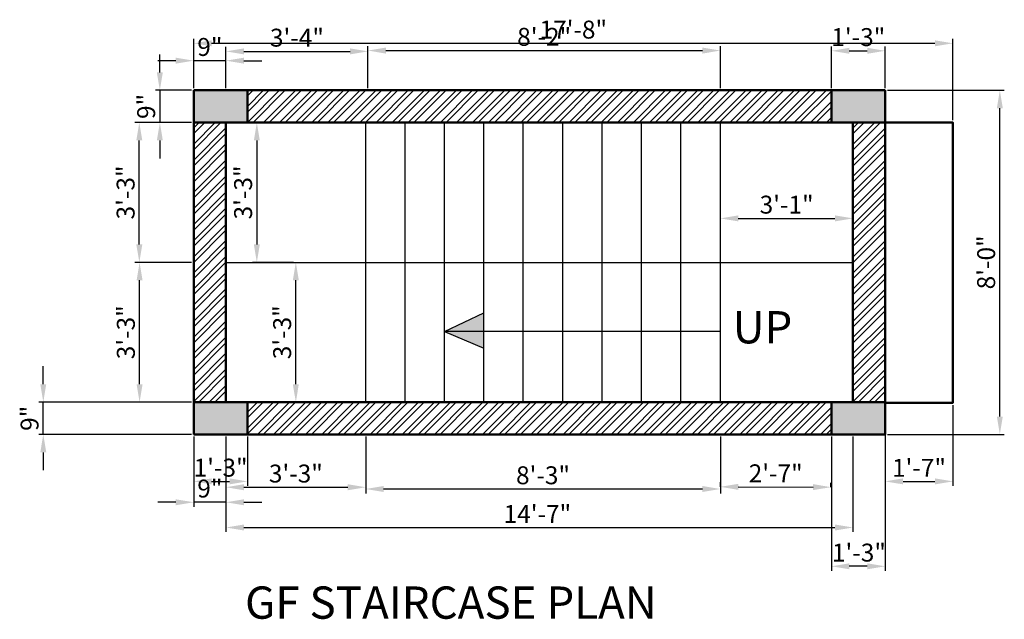
# Model space of a CAD drawing. Units: inches. Extents: x 1925 to 2200, y 918 to 1361.
# Tile 1 of 2: x 1925 to 2200, y 918 to 1085. Entities that reach past the tile are written whole.
import ezdxf

# ---------------------------------------------------------------- set-up
doc = ezdxf.new("R2010")
doc.units = ezdxf.units.IN
for name, color, linetype, lineweight in [('A-ANNO-DIMS', 2, 'Continuous', 18), ('A-ANNO-TEXT', 7, 'Continuous', 25), ('A-FLOR-STRS', 4, 'Continuous', 25), ('A-WALL', 7, 'Continuous', 50), ('A-WALL-PATT', 8, 'Continuous', 13), ('S-COLS-PATT', 1, 'Continuous', 13)]:
    doc.layers.add(name, color=color, linetype=linetype, lineweight=lineweight)
doc.styles.get("Standard").update_dxf_attribs({"font": 'arial.ttf'})
doc.dimstyles.new('ISO-25', dxfattribs={"dimtxt": 5, "dimasz": 5, "dimexe": 1.25, "dimexo": 0.625, "dimtad": 1, "dimdec": 0, "dimlunit": 3, "dimtxsty": 'Standard', "dimcen": 2.5, "dimadec": 0, "dimazin": 0, "dimtfac": 1, "dimtdec": 0, "dimtmove": 0, "dimatfit": 3, "dimfxl": 1, "dimarcsym": 0})
pattern_1 = [(45, (0, 0), (-2.245064, 2.245064), []), (45, (0, 1.5875), (-2.245064, 2.245064), [])]

# ---------------------------------------------------------------- blocks, each defined once
blk = doc.blocks.new('*D1')
at = {"layer": 'A-ANNO-DIMS', "color": 0, "lineweight": -2, "transparency": 16777216}
for p, q in [((2120.9, 1018.14), (2120.9, 1031.03)), ((2157.9, 1018.14), (2157.9, 1031.03)), ((2125.9, 1029.78), (2152.9, 1029.78))]:
    blk.add_line(p, q, dxfattribs=at)
at = {"layer": 'A-ANNO-DIMS', "color": 0, "transparency": 16777216}
for points in [[(2125.9, 1030.61), (2125.9, 1028.94), (2120.9, 1029.78)], [(2152.9, 1030.61), (2152.9, 1028.94), (2157.9, 1029.78)]]:
    blk.add_solid(points, dxfattribs=at)
at = {"layer": 'Defpoints', "color": 0, "transparency": 16777216}
for p in [(2157.9, 1029.78), (2120.9, 1017.51), (2157.9, 1017.51)]:
    blk.add_point(p, dxfattribs=at)
at = {"layer": 'A-ANNO-DIMS', "color": 0, "transparency": 16777216, "insert": (2139.4, 1032.96), "char_height": 5, "attachment_point": 5}
blk.add_mtext('3\'-1"', dxfattribs=at)
blk = doc.blocks.new('*D2')
at = {"layer": 'A-ANNO-DIMS', "color": 0, "lineweight": -2, "transparency": 16777216}
for p, q in [((1973.9, 1066.14), (1973.9, 1075.02)), ((1982.9, 1066.14), (1982.9, 1075.02)), ((1968.9, 1073.77), (1963.9, 1073.77)), ((1982.9, 1073.77), (1973.9, 1073.77)), ((1987.9, 1073.77), (1992.9, 1073.77))]:
    blk.add_line(p, q, dxfattribs=at)
at = {"layer": 'A-ANNO-DIMS', "color": 0, "transparency": 16777216}
for points in [[(1968.9, 1074.6), (1968.9, 1072.94), (1973.9, 1073.77)], [(1987.9, 1074.6), (1987.9, 1072.94), (1982.9, 1073.77)]]:
    blk.add_solid(points, dxfattribs=at)
at = {"layer": 'Defpoints', "color": 0, "transparency": 16777216}
for p in [(1973.9, 1073.77), (1973.9, 1065.51), (1982.9, 1065.51)]:
    blk.add_point(p, dxfattribs=at)
at = {"layer": 'A-ANNO-DIMS', "color": 0, "transparency": 16777216, "insert": (1978.4, 1076.95), "char_height": 5, "attachment_point": 5}
blk.add_mtext('9"', dxfattribs=at)
blk = doc.blocks.new('*D3')
at = {"layer": 'A-ANNO-DIMS', "color": 0, "lineweight": -2, "transparency": 16777216}
for p, q in [((1931.9, 983.51), (1931.9, 988.51)), ((1973.27, 978.51), (1930.65, 978.51)), ((1931.9, 969.51), (1931.9, 978.51)), ((1973.27, 969.51), (1930.65, 969.51)), ((1931.9, 964.51), (1931.9, 959.51))]:
    blk.add_line(p, q, dxfattribs=at)
at = {"layer": 'A-ANNO-DIMS', "color": 0, "transparency": 16777216}
for points in [[(1931.07, 983.51), (1932.73, 983.51), (1931.9, 978.51)], [(1931.07, 964.51), (1932.73, 964.51), (1931.9, 969.51)]]:
    blk.add_solid(points, dxfattribs=at)
at = {"layer": 'Defpoints', "color": 0, "transparency": 16777216}
for p in [(1931.9, 978.51), (1973.9, 978.51), (1973.9, 969.51)]:
    blk.add_point(p, dxfattribs=at)
at = {"layer": 'A-ANNO-DIMS', "color": 0, "transparency": 16777216, "insert": (1928.72, 974.01), "char_height": 5, "attachment_point": 5, "rotation": 90}
blk.add_mtext('9"', dxfattribs=at)
blk = doc.blocks.new('*D4')
at = {"layer": 'A-ANNO-DIMS', "color": 0, "lineweight": -2, "transparency": 16777216}
for p, q in [((1964.44, 1070.51), (1964.44, 1075.51)), ((1973.27, 1065.51), (1963.19, 1065.51)), ((1964.44, 1065.51), (1964.44, 1056.51)), ((1973.27, 1056.51), (1963.19, 1056.51)), ((1964.44, 1051.51), (1964.44, 1046.51))]:
    blk.add_line(p, q, dxfattribs=at)
at = {"layer": 'A-ANNO-DIMS', "color": 0, "transparency": 16777216}
for points in [[(1963.6, 1070.51), (1965.27, 1070.51), (1964.44, 1065.51)], [(1963.6, 1051.51), (1965.27, 1051.51), (1964.44, 1056.51)]]:
    blk.add_solid(points, dxfattribs=at)
at = {"layer": 'Defpoints', "color": 0, "transparency": 16777216}
for p in [(1973.9, 1065.51), (1964.44, 1056.51), (1973.9, 1056.51)]:
    blk.add_point(p, dxfattribs=at)
at = {"layer": 'A-ANNO-DIMS', "color": 0, "transparency": 16777216, "insert": (1961.26, 1061.01), "char_height": 5, "attachment_point": 5, "rotation": 90}
blk.add_mtext('9"', dxfattribs=at)
blk = doc.blocks.new('*D5')
at = {"layer": 'A-ANNO-DIMS', "color": 0, "lineweight": -2, "transparency": 16777216}
for p, q in [((1973.9, 968.89), (1973.9, 949.34)), ((1982.9, 968.89), (1982.9, 949.34)), ((1968.9, 950.59), (1963.9, 950.59)), ((1982.9, 950.59), (1973.9, 950.59)), ((1987.9, 950.59), (1992.9, 950.59))]:
    blk.add_line(p, q, dxfattribs=at)
at = {"layer": 'A-ANNO-DIMS', "color": 0, "transparency": 16777216}
for points in [[(1968.9, 951.42), (1968.9, 949.75), (1973.9, 950.59)], [(1987.9, 951.42), (1987.9, 949.75), (1982.9, 950.59)]]:
    blk.add_solid(points, dxfattribs=at)
at = {"layer": 'Defpoints', "color": 0, "transparency": 16777216}
for p in [(1973.9, 969.51), (1982.9, 969.51), (1973.9, 950.59)]:
    blk.add_point(p, dxfattribs=at)
at = {"layer": 'A-ANNO-DIMS', "color": 0, "transparency": 16777216, "insert": (1978.4, 953.77), "char_height": 5, "attachment_point": 5}
blk.add_mtext('9"', dxfattribs=at)
blk = doc.blocks.new('*D6')
at = {"layer": 'A-ANNO-DIMS', "color": 0, "lineweight": -2, "transparency": 16777216}
for p, q in [((1982.9, 968.89), (1982.9, 942.3)), ((2157.9, 968.89), (2157.9, 942.3)), ((1987.9, 943.55), (2152.9, 943.55))]:
    blk.add_line(p, q, dxfattribs=at)
at = {"layer": 'A-ANNO-DIMS', "color": 0, "transparency": 16777216}
for points in [[(1987.9, 944.38), (1987.9, 942.72), (1982.9, 943.55)], [(2152.9, 944.38), (2152.9, 942.72), (2157.9, 943.55)]]:
    blk.add_solid(points, dxfattribs=at)
at = {"layer": 'Defpoints', "color": 0, "transparency": 16777216}
for p in [(1982.9, 969.51), (2157.9, 969.51), (2157.9, 943.55)]:
    blk.add_point(p, dxfattribs=at)
at = {"layer": 'A-ANNO-DIMS', "color": 0, "transparency": 16777216, "insert": (2069.82, 946.68), "char_height": 5, "attachment_point": 5}
blk.add_mtext('14\'-7"', dxfattribs=at)
blk = doc.blocks.new('*D7')
at = {"layer": 'A-ANNO-DIMS', "color": 0, "lineweight": -2, "transparency": 16777216}
for p, q in [((1973.27, 1017.51), (1957.53, 1017.51)), ((1958.78, 983.51), (1958.78, 1012.51)), ((1973.27, 978.51), (1957.53, 978.51))]:
    blk.add_line(p, q, dxfattribs=at)
at = {"layer": 'A-ANNO-DIMS', "color": 0, "transparency": 16777216}
for points in [[(1957.95, 1012.51), (1959.61, 1012.51), (1958.78, 1017.51)], [(1957.95, 983.51), (1959.61, 983.51), (1958.78, 978.51)]]:
    blk.add_solid(points, dxfattribs=at)
at = {"layer": 'Defpoints', "color": 0, "transparency": 16777216}
for p in [(1958.78, 1017.51), (1973.9, 1017.51), (1973.9, 978.51)]:
    blk.add_point(p, dxfattribs=at)
at = {"layer": 'A-ANNO-DIMS', "color": 0, "transparency": 16777216, "insert": (1955.6, 998.01), "char_height": 5, "attachment_point": 5, "rotation": 90}
blk.add_mtext('3\'-3"', dxfattribs=at)
blk = doc.blocks.new('*D8')
at = {"layer": 'A-ANNO-DIMS', "color": 0, "lineweight": -2, "transparency": 16777216}
for p, q in [((1973.27, 1056.51), (1957.46, 1056.51)), ((1958.71, 1022.51), (1958.71, 1051.51)), ((1973.27, 1017.51), (1957.46, 1017.51))]:
    blk.add_line(p, q, dxfattribs=at)
at = {"layer": 'A-ANNO-DIMS', "color": 0, "transparency": 16777216}
for points in [[(1957.87, 1051.51), (1959.54, 1051.51), (1958.71, 1056.51)], [(1957.87, 1022.51), (1959.54, 1022.51), (1958.71, 1017.51)]]:
    blk.add_solid(points, dxfattribs=at)
at = {"layer": 'Defpoints', "color": 0, "transparency": 16777216}
for p in [(1958.71, 1056.51), (1973.9, 1056.51), (1973.9, 1017.51)]:
    blk.add_point(p, dxfattribs=at)
at = {"layer": 'A-ANNO-DIMS', "color": 0, "transparency": 16777216, "insert": (1955.53, 1037.01), "char_height": 5, "attachment_point": 5, "rotation": 90}
blk.add_mtext('3\'-3"', dxfattribs=at)
blk = doc.blocks.new('*D9')
at = {"layer": 'A-ANNO-DIMS', "color": 0, "lineweight": -2, "transparency": 16777216}
for p, q in [((1982.9, 1066.14), (1982.9, 1077.61)), ((2022.53, 1066.14), (2022.53, 1077.61)), ((1987.9, 1076.36), (2017.53, 1076.36))]:
    blk.add_line(p, q, dxfattribs=at)
at = {"layer": 'A-ANNO-DIMS', "color": 0, "transparency": 16777216}
for points in [[(1987.9, 1077.2), (1987.9, 1075.53), (1982.9, 1076.36)], [(2017.53, 1077.2), (2017.53, 1075.53), (2022.53, 1076.36)]]:
    blk.add_solid(points, dxfattribs=at)
at = {"layer": 'Defpoints', "color": 0, "transparency": 16777216}
for p in [(2022.53, 1076.36), (1982.9, 1065.51), (2022.53, 1065.51)]:
    blk.add_point(p, dxfattribs=at)
at = {"layer": 'A-ANNO-DIMS', "color": 0, "transparency": 16777216, "insert": (2002.71, 1079.54), "char_height": 5, "attachment_point": 5}
blk.add_mtext('3\'-4"', dxfattribs=at)
blk = doc.blocks.new('*D10')
at = {"layer": 'A-ANNO-DIMS', "color": 0, "lineweight": -2, "transparency": 16777216}
for p, q in [((2022.53, 1066.14), (2022.53, 1077.84)), ((2120.9, 1066.14), (2120.9, 1077.84)), ((2027.53, 1076.59), (2115.9, 1076.59))]:
    blk.add_line(p, q, dxfattribs=at)
at = {"layer": 'A-ANNO-DIMS', "color": 0, "transparency": 16777216}
for points in [[(2027.53, 1077.42), (2027.53, 1075.75), (2022.53, 1076.59)], [(2115.9, 1077.42), (2115.9, 1075.75), (2120.9, 1076.59)]]:
    blk.add_solid(points, dxfattribs=at)
at = {"layer": 'Defpoints', "color": 0, "transparency": 16777216}
for p in [(2120.9, 1076.59), (2022.53, 1065.51), (2120.9, 1065.51)]:
    blk.add_point(p, dxfattribs=at)
at = {"layer": 'A-ANNO-DIMS', "color": 0, "transparency": 16777216, "insert": (2071.71, 1079.77), "char_height": 5, "attachment_point": 5}
blk.add_mtext('8\'-2"', dxfattribs=at)
blk = doc.blocks.new('*D11')
at = {"layer": 'A-ANNO-DIMS', "color": 0, "lineweight": -2, "transparency": 16777216}
for p, q in [((2003.02, 1017.51), (2003.65, 1017.51)), ((2002.4, 983.51), (2002.4, 1012.51)), ((2003.02, 978.51), (2003.65, 978.51))]:
    blk.add_line(p, q, dxfattribs=at)
at = {"layer": 'A-ANNO-DIMS', "color": 0, "transparency": 16777216}
for points in [[(2001.56, 1012.51), (2003.23, 1012.51), (2002.4, 1017.51)], [(2001.56, 983.51), (2003.23, 983.51), (2002.4, 978.51)]]:
    blk.add_solid(points, dxfattribs=at)
at = {"layer": 'Defpoints', "color": 0, "transparency": 16777216}
for p in [(2002.4, 1017.51), (2002.4, 1017.51), (2002.4, 978.51)]:
    blk.add_point(p, dxfattribs=at)
at = {"layer": 'A-ANNO-DIMS', "color": 0, "transparency": 16777216, "insert": (1999.22, 998.01), "char_height": 5, "attachment_point": 5, "rotation": 90}
blk.add_mtext('3\'-3"', dxfattribs=at)
blk = doc.blocks.new('*D12')
at = {"layer": 'A-ANNO-DIMS', "color": 0, "lineweight": -2, "transparency": 16777216}
for p, q in [((2001.77, 1056.51), (1990.26, 1056.51)), ((1991.51, 1051.51), (1991.51, 1022.51)), ((2001.77, 1017.51), (1990.26, 1017.51))]:
    blk.add_line(p, q, dxfattribs=at)
at = {"layer": 'A-ANNO-DIMS', "color": 0, "transparency": 16777216}
for points in [[(1990.68, 1051.51), (1992.34, 1051.51), (1991.51, 1056.51)], [(1990.68, 1022.51), (1992.34, 1022.51), (1991.51, 1017.51)]]:
    blk.add_solid(points, dxfattribs=at)
at = {"layer": 'Defpoints', "color": 0, "transparency": 16777216}
for p in [(2002.4, 1056.51), (1991.51, 1017.51), (2002.4, 1017.51)]:
    blk.add_point(p, dxfattribs=at)
at = {"layer": 'A-ANNO-DIMS', "color": 0, "transparency": 16777216, "insert": (1988.33, 1037.01), "char_height": 5, "attachment_point": 5, "rotation": 90}
blk.add_mtext('3\'-3"', dxfattribs=at)
blk = doc.blocks.new('*D13')
at = {"layer": 'A-ANNO-DIMS', "color": 0, "lineweight": -2, "transparency": 16777216}
for p, q in [((2151.9, 1066.14), (2151.9, 1077.77)), ((2166.9, 1066.14), (2166.9, 1077.77)), ((2156.9, 1076.52), (2161.9, 1076.52))]:
    blk.add_line(p, q, dxfattribs=at)
at = {"layer": 'A-ANNO-DIMS', "color": 0, "transparency": 16777216}
for points in [[(2156.9, 1077.36), (2156.9, 1075.69), (2151.9, 1076.52)], [(2161.9, 1077.36), (2161.9, 1075.69), (2166.9, 1076.52)]]:
    blk.add_solid(points, dxfattribs=at)
at = {"layer": 'Defpoints', "color": 0, "transparency": 16777216}
for p in [(2166.9, 1076.52), (2151.9, 1065.51), (2166.9, 1065.51)]:
    blk.add_point(p, dxfattribs=at)
at = {"layer": 'A-ANNO-DIMS', "color": 0, "transparency": 16777216, "insert": (2159.4, 1079.7), "char_height": 5, "attachment_point": 5}
blk.add_mtext('1\'-3"', dxfattribs=at)
blk = doc.blocks.new('*D14')
at = {"layer": 'A-ANNO-DIMS', "color": 0, "lineweight": -2, "transparency": 16777216}
for p, q in [((2151.9, 968.89), (2151.9, 931.47)), ((2166.9, 968.89), (2166.9, 931.47)), ((2161.9, 932.72), (2156.9, 932.72))]:
    blk.add_line(p, q, dxfattribs=at)
at = {"layer": 'A-ANNO-DIMS', "color": 0, "transparency": 16777216}
for points in [[(2156.9, 933.56), (2156.9, 931.89), (2151.9, 932.72)], [(2161.9, 933.56), (2161.9, 931.89), (2166.9, 932.72)]]:
    blk.add_solid(points, dxfattribs=at)
at = {"layer": 'Defpoints', "color": 0, "transparency": 16777216}
for p in [(2151.9, 969.51), (2166.9, 969.51), (2151.9, 932.72)]:
    blk.add_point(p, dxfattribs=at)
at = {"layer": 'A-ANNO-DIMS', "color": 0, "transparency": 16777216, "insert": (2159.58, 935.9), "char_height": 5, "attachment_point": 5}
blk.add_mtext('1\'-3"', dxfattribs=at)
blk = doc.blocks.new('*D15')
at = {"layer": 'A-ANNO-DIMS', "color": 0, "lineweight": -2, "transparency": 16777216}
for p, q in [((1982.9, 968.89), (1982.9, 953.53)), ((2021.9, 968.89), (2021.9, 953.53)), ((1987.9, 954.78), (2016.9, 954.78))]:
    blk.add_line(p, q, dxfattribs=at)
at = {"layer": 'A-ANNO-DIMS', "color": 0, "transparency": 16777216}
for points in [[(1987.9, 955.61), (1987.9, 953.94), (1982.9, 954.78)], [(2016.9, 955.61), (2016.9, 953.94), (2021.9, 954.78)]]:
    blk.add_solid(points, dxfattribs=at)
at = {"layer": 'Defpoints', "color": 0, "transparency": 16777216}
for p in [(1982.9, 969.51), (2021.9, 969.51), (2021.9, 954.78)]:
    blk.add_point(p, dxfattribs=at)
at = {"layer": 'A-ANNO-DIMS', "color": 0, "transparency": 16777216, "insert": (2002.4, 957.95), "char_height": 5, "attachment_point": 5}
blk.add_mtext('3\'-3"', dxfattribs=at)
blk = doc.blocks.new('*D16')
at = {"layer": 'A-ANNO-DIMS', "color": 0, "lineweight": -2, "transparency": 16777216}
for p, q in [((2021.9, 968.89), (2021.9, 953.04)), ((2120.9, 968.89), (2120.9, 953.04)), ((2026.9, 954.29), (2115.9, 954.29))]:
    blk.add_line(p, q, dxfattribs=at)
at = {"layer": 'A-ANNO-DIMS', "color": 0, "transparency": 16777216}
for points in [[(2026.9, 955.12), (2026.9, 953.45), (2021.9, 954.29)], [(2115.9, 955.12), (2115.9, 953.45), (2120.9, 954.29)]]:
    blk.add_solid(points, dxfattribs=at)
at = {"layer": 'Defpoints', "color": 0, "transparency": 16777216}
for p in [(2021.9, 969.51), (2120.9, 969.51), (2120.9, 954.29)]:
    blk.add_point(p, dxfattribs=at)
at = {"layer": 'A-ANNO-DIMS', "color": 0, "transparency": 16777216, "insert": (2071.4, 957.47), "char_height": 5, "attachment_point": 5}
blk.add_mtext('8\'-3"', dxfattribs=at)
blk = doc.blocks.new('*D17')
at = {"layer": 'A-ANNO-DIMS', "color": 0, "lineweight": -2, "transparency": 16777216}
for p, q in [((2120.9, 954.91), (2120.9, 956.15)), ((2125.9, 954.88), (2146.77, 954.82)), ((2151.77, 954.81), (2151.77, 956.05))]:
    blk.add_line(p, q, dxfattribs=at)
at = {"layer": 'A-ANNO-DIMS', "color": 0, "transparency": 16777216}
for points in [[(2125.9, 955.72), (2125.89, 954.05), (2120.9, 954.9)], [(2146.77, 955.65), (2146.77, 953.98), (2151.77, 954.8)]]:
    blk.add_solid(points, dxfattribs=at)
at = {"layer": 'Defpoints', "color": 0, "transparency": 16777216}
for p in [(2120.9, 954.29), (2151.77, 954.8), (2151.77, 954.19)]:
    blk.add_point(p, dxfattribs=at)
at = {"layer": 'A-ANNO-DIMS', "color": 0, "transparency": 16777216, "insert": (2136.34, 957.99), "char_height": 5, "attachment_point": 5, "rotation": 359.8217}
blk.add_mtext('2\'-7"', dxfattribs=at)
blk = doc.blocks.new('*D38')
at = {"layer": 'A-ANNO-DIMS', "color": 0, "lineweight": -2, "transparency": 16777216}
for p, q in [((1973.9, 1066.14), (1973.9, 1079.86)), ((1978.9, 1078.61), (2180.81, 1078.61)), ((2185.81, 1057.14), (2185.81, 1079.86))]:
    blk.add_line(p, q, dxfattribs=at)
at = {"layer": 'A-ANNO-DIMS', "color": 0, "transparency": 16777216}
for points in [[(1978.9, 1079.45), (1978.9, 1077.78), (1973.9, 1078.61)], [(2180.81, 1079.45), (2180.81, 1077.78), (2185.81, 1078.61)]]:
    blk.add_solid(points, dxfattribs=at)
at = {"layer": 'Defpoints', "color": 0, "transparency": 16777216}
for p in [(2185.81, 1078.61), (1973.9, 1065.51), (2185.81, 1056.51)]:
    blk.add_point(p, dxfattribs=at)
at = {"layer": 'A-ANNO-DIMS', "color": 0, "transparency": 16777216, "insert": (2079.85, 1081.79), "char_height": 5, "attachment_point": 5}
blk.add_mtext('17\'-8"', dxfattribs=at)
blk = doc.blocks.new('*D39')
at = {"layer": 'A-ANNO-DIMS', "color": 0, "lineweight": -2, "transparency": 16777216}
for p, q in [((2167.52, 1065.51), (2200.16, 1065.51)), ((2198.91, 974.51), (2198.91, 1060.51)), ((2167.52, 969.51), (2200.16, 969.51))]:
    blk.add_line(p, q, dxfattribs=at)
at = {"layer": 'A-ANNO-DIMS', "color": 0, "transparency": 16777216}
for points in [[(2198.08, 1060.51), (2199.74, 1060.51), (2198.91, 1065.51)], [(2198.08, 974.51), (2199.74, 974.51), (2198.91, 969.51)]]:
    blk.add_solid(points, dxfattribs=at)
at = {"layer": 'Defpoints', "color": 0, "transparency": 16777216}
for p in [(2166.9, 1065.51), (2198.91, 1065.51), (2166.9, 969.51)]:
    blk.add_point(p, dxfattribs=at)
at = {"layer": 'A-ANNO-DIMS', "color": 0, "transparency": 16777216, "insert": (2195.73, 1017.51), "char_height": 5, "attachment_point": 5, "rotation": 90}
blk.add_mtext('8\'-0"', dxfattribs=at)
blk = doc.blocks.new('*D40')
at = {"layer": 'A-ANNO-DIMS', "color": 0, "lineweight": -2, "transparency": 16777216}
for p, q in [((2166.9, 977.89), (2166.9, 955.16)), ((2185.81, 977.71), (2185.81, 955.16)), ((2171.9, 956.41), (2180.81, 956.41))]:
    blk.add_line(p, q, dxfattribs=at)
at = {"layer": 'A-ANNO-DIMS', "color": 0, "transparency": 16777216}
for points in [[(2171.9, 957.25), (2171.9, 955.58), (2166.9, 956.41)], [(2180.81, 957.25), (2180.81, 955.58), (2185.81, 956.41)]]:
    blk.add_solid(points, dxfattribs=at)
at = {"layer": 'Defpoints', "color": 0, "transparency": 16777216}
for p in [(2166.9, 978.51), (2185.81, 978.33), (2185.81, 956.41)]:
    blk.add_point(p, dxfattribs=at)
at = {"layer": 'A-ANNO-DIMS', "color": 0, "transparency": 16777216, "insert": (2176.35, 959.55), "char_height": 5, "attachment_point": 5}
blk.add_mtext('1\'-7"', dxfattribs=at)
blk = doc.blocks.new('*D41')
at = {"layer": 'A-ANNO-DIMS', "color": 0, "lineweight": -2, "transparency": 16777216}
for p, q in [((1973.9, 968.89), (1973.9, 955.16)), ((1988.9, 968.89), (1988.9, 955.16)), ((1978.9, 956.41), (1983.9, 956.41))]:
    blk.add_line(p, q, dxfattribs=at)
at = {"layer": 'A-ANNO-DIMS', "color": 0, "transparency": 16777216}
for points in [[(1978.9, 957.25), (1978.9, 955.58), (1973.9, 956.41)], [(1983.9, 957.25), (1983.9, 955.58), (1988.9, 956.41)]]:
    blk.add_solid(points, dxfattribs=at)
at = {"layer": 'Defpoints', "color": 0, "transparency": 16777216}
for p in [(1973.9, 969.51), (1988.9, 969.51), (1988.9, 956.41)]:
    blk.add_point(p, dxfattribs=at)
at = {"layer": 'A-ANNO-DIMS', "color": 0, "transparency": 16777216, "insert": (1981.4, 959.59), "char_height": 5, "attachment_point": 5}
blk.add_mtext('1\'-3"', dxfattribs=at)

msp = doc.modelspace()

# ---------------------------------------------------------------- hatches: boundary and pattern name
at = {"layer": 'A-WALL-PATT'}
h = msp.add_hatch(dxfattribs=at)
h.set_pattern_fill('STEEL', color=256)
h.set_pattern_definition(pattern_1)
h.paths.add_polyline_path([(2151.9, 1056.51), (2151.9, 1065.51), (1988.9, 1065.51), (1988.9, 1056.51)])
h = msp.add_hatch(dxfattribs=at)
h.set_pattern_fill('STEEL', color=256)
h.set_pattern_definition(pattern_1)
h.paths.add_polyline_path([(1982.9, 1056.51), (1973.9, 1056.51), (1973.9, 978.51), (1982.9, 978.51)])
h = msp.add_hatch(dxfattribs=at)
h.set_pattern_fill('STEEL', color=256)
h.set_pattern_definition(pattern_1)
h.paths.add_polyline_path([(2157.9, 978.51), (2166.9, 978.51), (2166.9, 1056.51), (2157.9, 1056.51)])
h = msp.add_hatch(color=256, dxfattribs=at)
h.dxf.hatch_style = 1
h.paths.add_polyline_path([(2043.9, 998.23), (2054.9, 998.23), (2054.9, 1003.4)])
h = msp.add_hatch(color=256, dxfattribs=at)
h.dxf.hatch_style = 1
h.paths.add_polyline_path([(2043.9, 998.23), (2054.9, 993.57), (2054.9, 998.23)])
h = msp.add_hatch(dxfattribs=at)
h.set_pattern_fill('STEEL', color=256)
h.set_pattern_definition(pattern_1)
h.paths.add_polyline_path([(2151.9, 969.51), (2151.9, 978.51), (2120.9, 978.51), (2021.9, 978.51), (1988.9, 978.51), (1988.9, 969.51), (2021.9, 969.51), (2120.9, 969.51)])
at = {"layer": 'S-COLS-PATT'}
h = msp.add_hatch(color=256, dxfattribs=at)
h.dxf.hatch_style = 1
h.paths.add_polyline_path([(1988.9, 1056.51), (1988.9, 1065.51), (1973.9, 1065.51), (1973.9, 1056.51)])
h = msp.add_hatch(color=256, dxfattribs=at)
h.dxf.hatch_style = 1
h.paths.add_polyline_path([(2151.9, 1065.51), (2151.9, 1056.51), (2166.9, 1056.51), (2166.9, 1065.51)])
h = msp.add_hatch(color=256, dxfattribs=at)
h.dxf.hatch_style = 1
h.paths.add_polyline_path([(1982.9, 969.51), (1988.9, 969.51), (1988.9, 978.51), (1982.9, 978.51), (1973.9, 978.51), (1973.9, 969.51)])
h = msp.add_hatch(color=256, dxfattribs=at)
h.dxf.hatch_style = 1
h.paths.add_polyline_path([(2166.9, 969.51), (2166.9, 978.51), (2151.9, 978.51), (2151.9, 969.51)])

# ---------------------------------------------------------------- linework, layer by layer
at = {"layer": 'A-FLOR-STRS'}
for p, q in [((2021.9, 978.51), (2021.9, 1056.51)), ((2032.9, 978.51), (2032.9, 1056.51)), ((2043.9, 978.51), (2043.9, 1056.51)), ((2054.9, 978.51), (2054.9, 1056.51)), ((2065.9, 978.51), (2065.9, 1056.51)), ((2076.9, 978.51), (2076.9, 1056.51)), ((2087.9, 978.51), (2087.9, 1056.51)), ((2098.9, 978.51), (2098.9, 1056.51)), ((2109.9, 978.51), (2109.9, 1056.51)), ((2120.9, 978.51), (2120.9, 1056.51)), ((1982.9, 1017.51), (2021.9, 1017.51)), ((1982.9, 1017.51), (2157.9, 1017.51)), ((2043.9, 998.23), (2054.9, 1003.4)), ((2054.9, 993.57), (2054.9, 1003.4)), ((2120.9, 998.23), (2043.9, 998.23)), ((2043.9, 998.23), (2054.9, 993.57))]:
    msp.add_line(p, q, dxfattribs=at)
at = {"layer": 'A-WALL'}
for p, q in [((1973.9, 969.51), (1973.9, 1065.51)), ((1973.9, 1065.51), (2166.9, 1065.51)), ((1988.9, 1056.51), (1988.9, 1065.51)), ((2151.9, 1065.51), (2151.9, 1056.51)), ((2166.9, 1065.51), (2166.9, 969.51)), ((1973.9, 1056.51), (2166.9, 1056.51)), ((1982.9, 978.51), (1982.9, 1056.51)), ((2157.9, 1056.51), (2157.9, 978.51)), ((1973.9, 978.51), (1982.9, 978.51)), ((1982.9, 978.51), (2021.9, 978.51)), ((1988.9, 969.51), (1988.9, 978.51)), ((2021.9, 978.51), (2120.9, 978.51)), ((2120.9, 978.51), (2151.9, 978.51)), ((2151.9, 978.51), (2166.9, 978.51)), ((2151.9, 978.51), (2151.9, 969.51)), ((1973.9, 969.51), (1982.9, 969.51)), ((1982.9, 969.51), (2021.9, 969.51)), ((2021.9, 969.51), (2120.9, 969.51)), ((2120.9, 969.51), (2151.9, 969.51)), ((2151.9, 969.51), (2166.9, 969.51))]:
    msp.add_line(p, q, dxfattribs=at)
for points in [[(2166.9, 1056.51), (2166.9, 1056.51), (2166.9, 978.51), (2166.9, 978.51)], [(2166.9, 1056.51), (2185.81, 1056.51), (2185.81, 978.33), (2166.9, 978.33)]]:
    msp.add_lwpolyline(points, close=True, dxfattribs=at)

# ---------------------------------------------------------------- texts
at = {"layer": 'A-ANNO-TEXT', "char_height": 9, "attachment_point": 1}
for s, width, insert in [('{\\fArial|b1|i0|c0|p34;UP}', 18.9712, (2124.35, 1003.91)), ('{\\fArial|b1|i0|c0|p34;GF STAIRCASE PLAN}', 139.1979, (1988.22, 927.1))]:
    msp.add_mtext_dynamic_manual_height_columns(s, width=width, gutter_width=12.5, heights=[0], dxfattribs=dict(at, insert=insert))

# ---------------------------------------------------------------- dimensions: what is measured, and where the dimension line sits
at = {"layer": 'A-ANNO-DIMS'}
for base, p1, p2, override, picture, middle in [((2185.81, 1078.61), (1973.9, 1065.51), (2185.81, 1056.51), {"dimdec": 1, "dimlfac": 1, "dimrnd": 0, "dimzin": 1, "dimdsep": 46, "dimlunit": 4, "dimfrac": 2}, '*D38', (2079.85, 1081.79)), ((2022.53, 1076.36), (1982.9, 1065.51), (2022.53, 1065.51), {"dimclrd": 0, "dimclre": 0, "dimclrt": 0}, '*D9', (2002.71, 1079.54)), ((2120.9, 1076.59), (2022.53, 1065.51), (2120.9, 1065.51), {"dimclrd": 0, "dimclre": 0, "dimclrt": 0}, '*D10', (2071.71, 1079.77)), ((2166.9, 1076.52), (2151.9, 1065.51), (2166.9, 1065.51), {"dimclrd": 0, "dimclre": 0, "dimclrt": 0}, '*D13', (2159.4, 1079.7)), ((1973.9, 1073.77), (1982.9, 1065.51), (1973.9, 1065.51), {"dimclrd": 0, "dimclre": 0, "dimclrt": 0}, '*D2', (1978.4, 1076.95)), ((2157.9, 1029.78), (2120.9, 1017.51), (2157.9, 1017.51), {"dimclrd": 0, "dimclre": 0, "dimclrt": 0}, '*D1', (2139.4, 1032.96)), ((2185.81, 956.41), (2166.9, 978.51), (2185.81, 978.33), {"dimdec": 1, "dimlfac": 1, "dimrnd": 0, "dimzin": 1, "dimdsep": 46, "dimlunit": 4, "dimfrac": 2}, '*D40', (2176.35, 959.55)), ((1973.9, 950.59), (1982.9, 969.51), (1973.9, 969.51), {"dimclrd": 0, "dimclre": 0, "dimclrt": 0}, '*D5', (1978.4, 953.77)), ((1988.9, 956.41), (1973.9, 969.51), (1988.9, 969.51), {"dimdec": 1, "dimlfac": 1, "dimrnd": 0, "dimzin": 1, "dimdsep": 46, "dimlunit": 4, "dimfrac": 2}, '*D41', (1981.4, 959.59)), ((2021.9, 954.78), (1982.9, 969.51), (2021.9, 969.51), {"dimclrd": 0, "dimclre": 0, "dimclrt": 0}, '*D15', (2002.4, 957.95)), ((2120.9, 954.29), (2021.9, 969.51), (2120.9, 969.51), {"dimclrd": 0, "dimclre": 0, "dimclrt": 0}, '*D16', (2071.4, 957.47))]:
    dim = msp.add_linear_dim(base=base, p1=p1, p2=p2, dimstyle='ISO-25', override=override, dxfattribs=at)
    dim.commit()
    dim.dimension.update_dxf_attribs({"geometry": picture, "text_midpoint": middle})
for p1, p2, distance, picture, middle in [((1973.9, 1065.51), (1973.9, 1056.51), -9.46, '*D4', (1961.26, 1061.01)), ((2120.9, 954.29), (2151.77, 954.19), 0.61, '*D17', (2136.34, 957.99))]:
    dim = msp.add_aligned_dim(p1=p1, p2=p2, distance=distance, dimstyle='ISO-25', override={"dimclrd": 0, "dimclre": 0, "dimclrt": 0}, dxfattribs=at)
    dim.commit()
    dim.dimension.update_dxf_attribs({"geometry": picture, "text_midpoint": middle})
for base, p1, p2, override, picture, middle in [((2198.91, 1065.51), (2166.9, 969.51), (2166.9, 1065.51), {"dimdec": 1, "dimlfac": 1, "dimrnd": 0, "dimzin": 1, "dimdsep": 46, "dimlunit": 4, "dimfrac": 2}, '*D39', (2195.73, 1017.51)), ((1958.71, 1056.51), (1973.9, 1017.51), (1973.9, 1056.51), {"dimclrd": 0, "dimclre": 0, "dimclrt": 0}, '*D8', (1955.53, 1037.01)), ((1991.51, 1017.51), (2002.4, 1056.51), (2002.4, 1017.51), {"dimclrd": 0, "dimclre": 0, "dimclrt": 0}, '*D12', (1988.33, 1037.01)), ((1958.78, 1017.51), (1973.9, 978.51), (1973.9, 1017.51), {"dimclrd": 0, "dimclre": 0, "dimclrt": 0}, '*D7', (1955.6, 998.01)), ((2002.4, 1017.51), (2002.4, 978.51), (2002.4, 1017.51), {"dimclrd": 0, "dimclre": 0, "dimclrt": 0}, '*D11', (1999.22, 998.01)), ((1931.9, 978.51), (1973.9, 969.51), (1973.9, 978.51), {"dimclrd": 0, "dimclre": 0, "dimclrt": 0}, '*D3', (1928.72, 974.01))]:
    dim = msp.add_linear_dim(base=base, p1=p1, p2=p2, angle=90, dimstyle='ISO-25', override=override, dxfattribs=at)
    dim.commit()
    dim.dimension.update_dxf_attribs({"geometry": picture, "text_midpoint": middle})
for base, p1, p2, picture, middle in [((2157.9, 943.55), (1982.9, 969.51), (2157.9, 969.51), '*D6', (2069.82, 943.55)), ((2151.9, 932.72), (2166.9, 969.51), (2151.9, 969.51), '*D14', (2159.58, 932.72))]:
    dim = msp.add_linear_dim(base=base, p1=p1, p2=p2, dimstyle='ISO-25', override={"dimclrd": 0, "dimclre": 0, "dimclrt": 0}, dxfattribs=at)
    dim.commit()
    dim.dimension.update_dxf_attribs({"geometry": picture, "text_midpoint": middle, "dimtype": 160})

doc.saveas('drawing.dxf')
